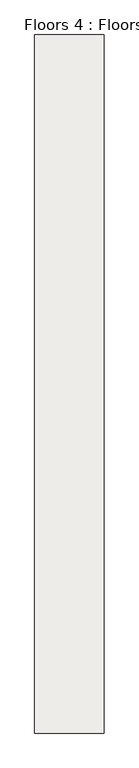
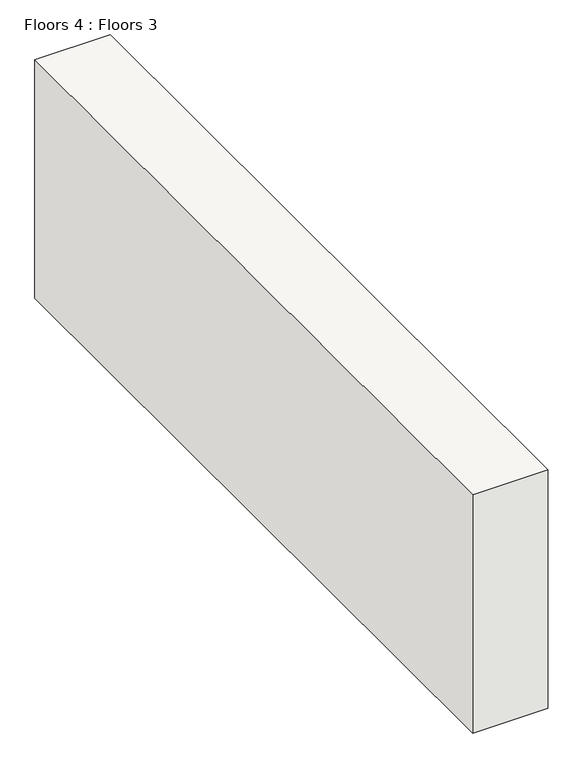
"""IFC4 building model written with IfcOpenShell, lengths in millimetres: slab geometry, Floors 4 : Floors 3."""

from ifc_helpers import new_model, si_unit, frame, origin, place, context, project, spatial, polyline, outline, extrude, source, transform, mapped, element, save


def floors_4_floors_3_d07f1cc1(model_context):
    return source(origin(), model_context, "Body", "SweptSolid", [
        extrude(outline(polyline([(-22.6504261, -2226.6675594), (-205.0528935, -2226.6675594), (-205.0528935, -394.0464931), (-22.6504261, -394.0464931), (-22.6504261, -2226.6675594)])), frame((0.0, 0.0, 8534.4), z_axis=(0.0, 0.0, 1.0), x_axis=(1.0, 0.0, 0.0)), (0.0, 0.0, 1.0), 609.529249),
    ])


if __name__ == "__main__":
    model = new_model("IFC4")
    model_context = context("Model", 3, world=origin())
    ifc_project = project(units=[si_unit("LENGTHUNIT", "METRE", prefix="MILLI")], contexts=[model_context])
    site = spatial("IfcSite", under=ifc_project)
    building = spatial("IfcBuilding", under=site)
    placement = place(None, origin())
    floors_4_floors_3_shape = floors_4_floors_3_d07f1cc1(model_context)
    element("IfcSlab", 1, ObjectType="Floors 4 : Floors 3", at=placement, inside=building, context=model_context, shape_type="MappedRepresentation", body=[
        mapped(floors_4_floors_3_shape, transform((0.0, 0.0, 0.0), x_axis=(1.0, 0.0, 0.0), y_axis=(0.0, 1.0, 0.0), z_axis=(0.0, 0.0, 1.0))),
    ])
    save(model, "model.ifc")

# Revit data of these elements
# Element 1 (IfcSlab, "Floors 4 : Floors 3")
#   Materials on its faces: "Default Floor"
# Materials
#   "Default Floor": colour RGB 128 128 128, transparency 0, Cost = 0
